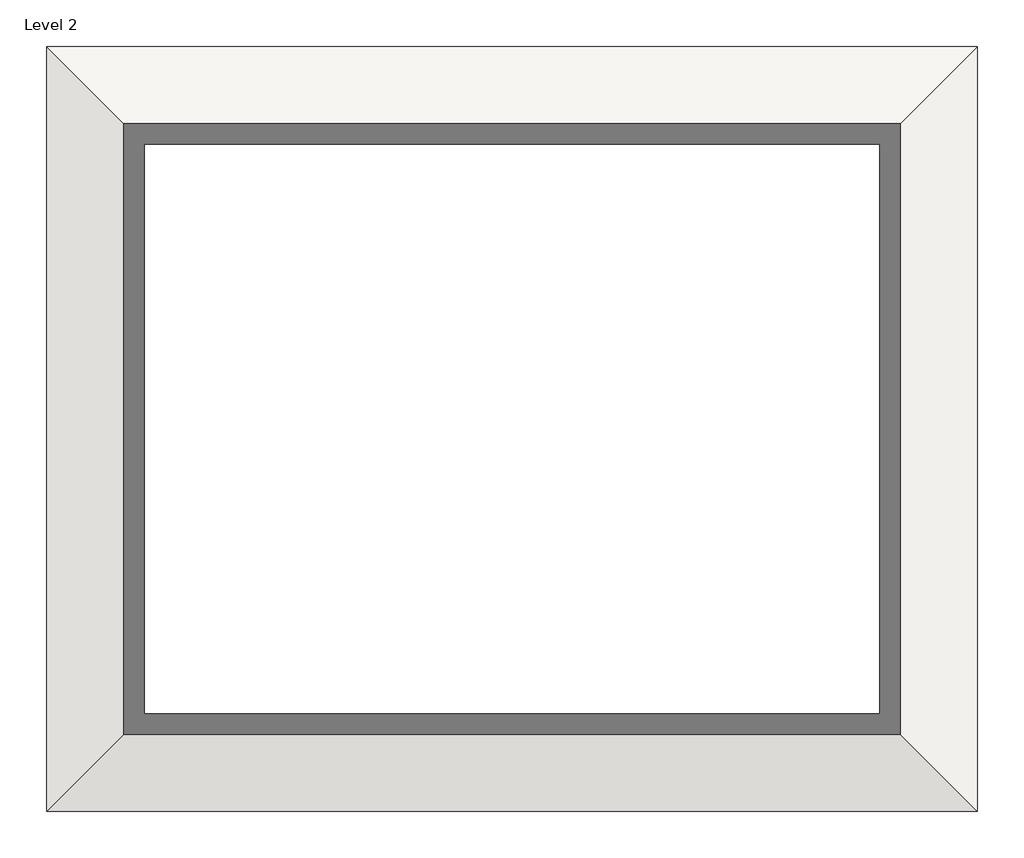
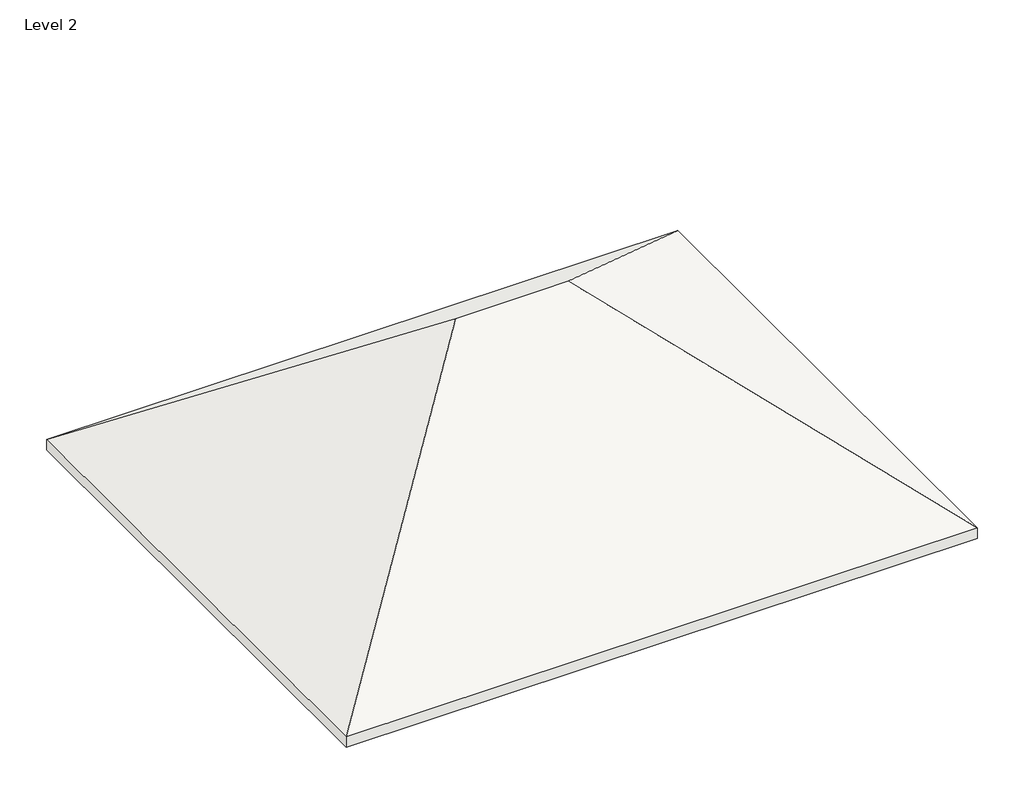
# One storey: 1 roof.
"""IFC4 building model written with IfcOpenShell, lengths in millimetres."""

from ifc_helpers import new_model, si_unit, origin, place, context, project, spatial, faceted_brep, element, save

model = new_model("IFC4")

# Units and contexts
model_context = context("Model", 3, world=origin())
ifc_project = project(units=[si_unit("LENGTHUNIT", "METRE", prefix="MILLI")], contexts=[model_context])

# Site, building, storey
site = spatial("IfcSite", under=ifc_project)
building = spatial("IfcBuilding", under=site)
storey = spatial("IfcBuildingStorey", under=building, Name="Level 2", Elevation=3048.0)

# Roof
placement = place(None, origin())
element("IfcRoof", 1, ObjectType="Wood Rafter 8\" - Asphalt Shingle - Insulated", at=placement, inside=storey, context=model_context, shape_type="Brep", body=[
    faceted_brep([(1827.204801, 6956.5076725, 3048.0), (-4395.795199, 733.5076725, 7715.25), (-7088.195199, 733.5076725, 7715.25), (-13311.195199, 6956.5076725, 3048.0), (1827.204801, -5489.4923275, 3048.0), (-13311.195199, -5489.4923275, 3048.0), (1827.204801, 6956.5076725, 3313.90625), (-13311.195199, 6956.5076725, 3313.90625), (-7088.195199, 733.5076725, 7981.15625), (-4395.795199, 733.5076725, 7981.15625), (1827.204801, -5489.4923275, 3313.90625), (-13311.195199, -5489.4923275, 3313.90625)], [[[0, 1, 2, 3]], [[1, 0, 4]], [[5, 2, 1, 4]], [[3, 2, 5]], [[6, 7, 8, 9]], [[6, 9, 10]], [[11, 10, 9, 8]], [[7, 11, 8]], [[3, 7, 6, 0]], [[5, 11, 7, 3]], [[4, 10, 11, 5]], [[0, 6, 10, 4]]]),
])

save(model, "model.ifc")

# Revit data of these elements
# Type "Wood Rafter 8\" - Asphalt Shingle - Insulated"
#   Assembly Code = "B1020"
#   Layers, outside or top first: 0' - 0 1/4" "Asphalt Shingle" (function 4); 0' - 0 5/8" "Plywood, Sheathing" (function 2); 0' - 7 1/2" "Structure, Wood Joist/Rafter Layer, Batt Insulation" (function 1)
# Element 1 (IfcRoof, "Wood Rafter 8\" - Asphalt Shingle - Insulated")
#   built-in parameter 1001705 = 26.1849 (stored number, unit not read)
#   built-in parameter 1001710 = 33615
#   Phase Created = New Construction
#   Materials on its faces: "Structure, Wood Joist/Rafter Layer, Batt Insulation", "Asphalt Shingle"
# Materials
#   "Asphalt Shingle": class "Generic", colour RGB 155 155 155, transparency 0, Description = "Asphalt roofing shingle", Cost = 0
#   "Plywood, Sheathing": class "Wood", colour RGB 212 179 113, transparency 0, Description = "Plywood, sheathing grade", Cost = 0
#   "Structure, Wood Joist/Rafter Layer, Batt Insulation": class "Wood", colour RGB 127 127 127, transparency 0, Description = "Wood framing, insulated", Cost = 0
